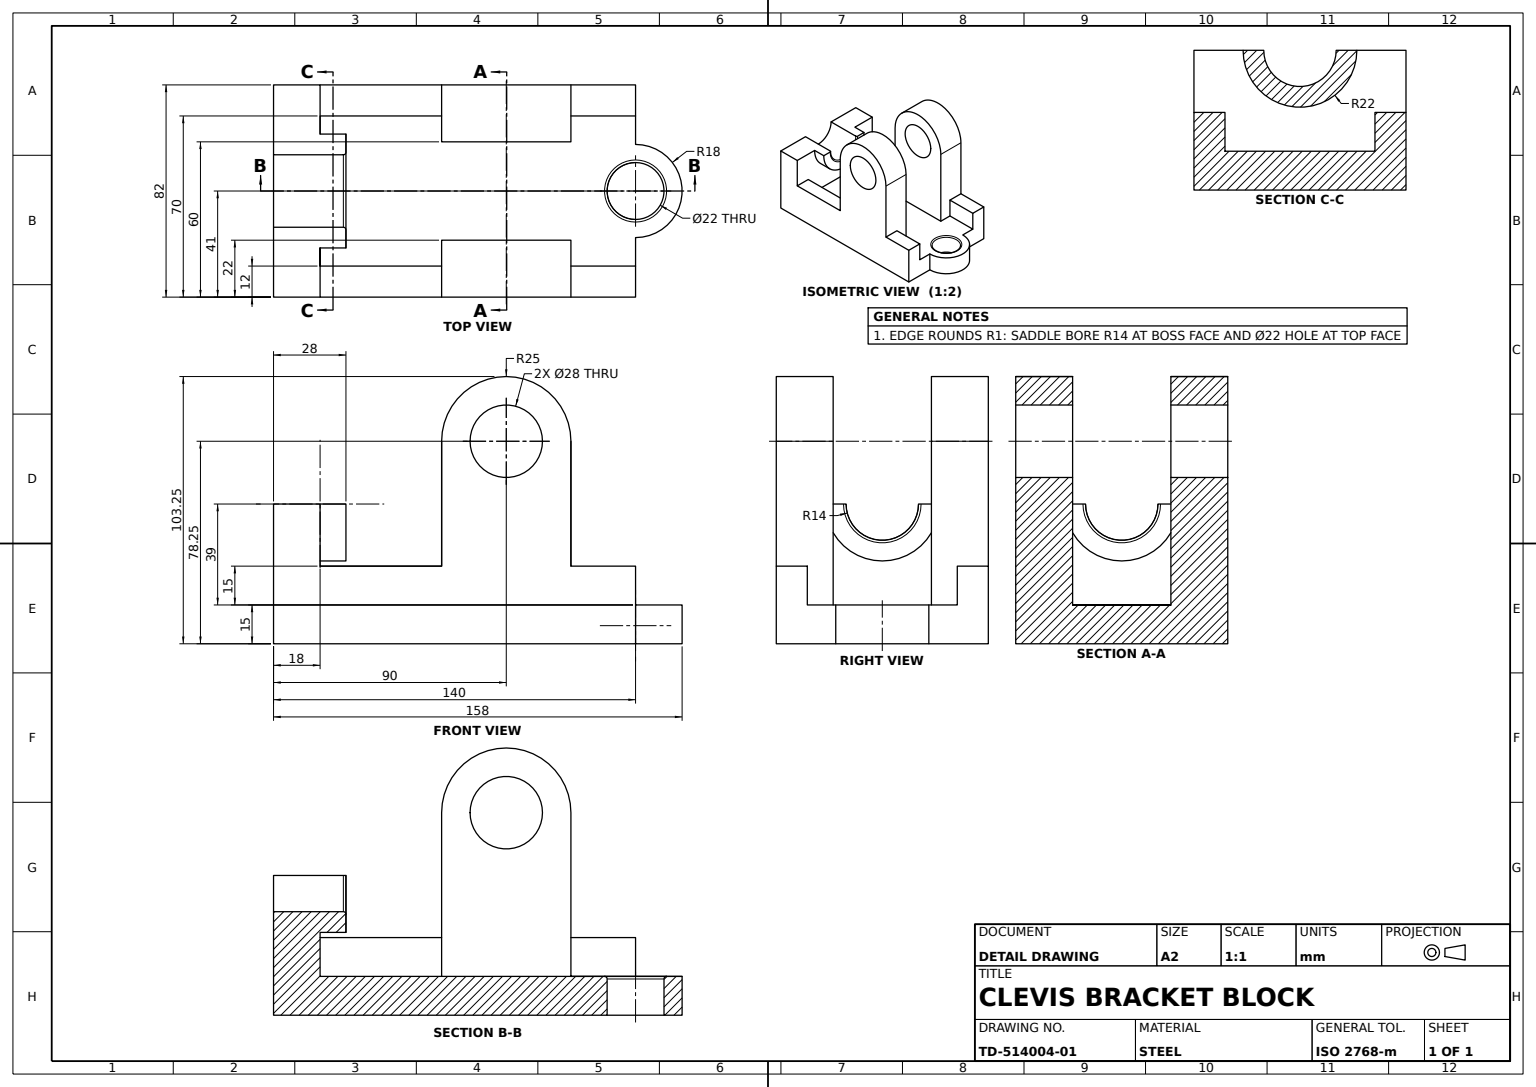
SolidWorks part; units mm, degrees
material "Plain Carbon Steel"
ref_plane "Front Plane" through (0, 0, 0) normal (0, 0, 1) x (1, 0, 0)
ref_plane "Top Plane" through (0, 0, 0) normal (0, 1, 0) x (1, 0, 0)
ref_plane "Right Plane" through (0, 0, 0) normal (1, 0, 0) x (0, 0, -1)
sketch "Base Plate Sketch" plane through (0, 0, 0) normal (0, 1, 0) x (1, 0, 0)
  line L0 (70, -18) -> (70, -41)
  line L1 (-70, 41) -> (70, 41)
  line L2 (-70, 41) -> (-70, -41)
  line L3 (-70, -41) -> (70, -41)
  line L4 (70, 41) -> (70, 18)
  line L5 (-70, 41) -> (70, -41) construction
  line L6 (-70, -41) -> (70, 41) construction
  arc A0 (70, -18) -> (70, 18) centre (70, 0) ccw
  circle A1 centre (70, 0) radius 11
  point P0 (0, 0)
  dimension "D3" = 36
  dimension "D4" = 22
  dimension "D1" = 82
  dimension "D2" = 140
  dimension "D5" = 23
  dimension "D6" = 41
extrude "Base Plate" add sketch "Base Plate Sketch" along normal blind 15
sketch "Rear Wall Sketch" plane through (0, 15, 0) normal (0, 1, 0) x (1, 0, 0)
  line L0 (-70, -41) -> (70, -41) construction
  line L1 (-70, 41) -> (-52, 41)
  line L2 (-70, 41) -> (-70, -41)
  line L3 (-70, -41) -> (-52, -41)
  line L4 (-52, 41) -> (-52, -41)
  dimension "D1" = 18
extrude "Rear Wall" add sketch "Rear Wall Sketch" along normal blind 39
sketch "Step Blocks Sketch" plane through (0, 15, 0) normal (0, 1, 0) x (1, 0, 0)
  line L0 (70, 18) -> (70, 41) construction
  line L1 (-52, 41) -> (70, 41)
  line L2 (-52, 41) -> (-52, 29)
  line L3 (-52, 29) -> (70, 29)
  line L4 (70, 41) -> (70, 29)
  line L5 (70, -41) -> (70, -18) construction
  line L6 (-52, -41) -> (70, -41)
  line L7 (-52, -41) -> (-52, -29)
  line L8 (-52, -29) -> (70, -29)
  line L9 (70, -41) -> (70, -29)
  dimension "D1" = 12
  dimension "D2" = 12
extrude "Step Blocks" add sketch "Step Blocks Sketch" along normal blind 15
sketch "Bearing Ear 1 Sketch" plane through (0, 0, 41) normal (0, 0, 1) x (1, 0, 0)
  line L0 (-70, 54) -> (-70, 0) construction
  line L4 (-5, 78.2548) -> (-5, 30)
  line L5 (-52, 30) -> (70, 30) construction
  line L6 (45, 78.2548) -> (45, 30)
  line L8 (-70, 0) -> (70, 0) construction
  line L9 (-5, 30) -> (-5, 0)
  line L10 (-5, 0) -> (45, 0)
  line L11 (45, 0) -> (45, 30)
  circle A0 centre (20, 78.2548) radius 14
  arc A1 (45, 78.2548) -> (-5, 78.2548) centre (20, 78.2548) ccw
  dimension "D1" = 28
  dimension "D2" = 50
  dimension "D3" = 90
  dimension "D4" = 78.2548
extrude "Bearing Ear 1" add sketch "Bearing Ear 1 Sketch" against normal blind 22
sketch "Bearing Ear 2 Sketch" plane through (0, 0, -41) normal (0, 0, -1) x (-1, 0, 0)
  line L0 (-45, 78.2548) -> (-45, 0)
  line L3 (-45, 0) -> (5, 0)
  line L4 (-70, 0) -> (70, 0) construction
  line L5 (5, 0) -> (5, 78.2548)
  circle A0 centre (-20, 78.2548) radius 14
  arc A1 (-45, 78.2548) -> (5, 78.2548) centre (-20, 78.2548) cw
  dimension "D1" = 25
  dimension "D2" = 28
  dimension "D3" = 78.2548
  dimension "D4" = 50
extrude "Bearing Ear 2" add sketch "Bearing Ear 2 Sketch" against normal blind 22
sketch "Saddle Cut Sketch" plane through (-70, 0, 0) normal (-1, 0, 0) x (0, 0, 1)
  line L0 (-41, 54) -> (41, 54) construction
  line L1 (-14, 54) -> (14, 54)
  arc A0 (-14, 54) -> (14, 54) centre (0, 54) ccw
  dimension "D1" = 14
extrude "Saddle Cut" cut sketch "Saddle Cut Sketch" against normal blind 22
sketch "Saddle Boss Sketch" plane through (-70, 0, 0) normal (-1, 0, 0) x (0, 0, 1)
  line L0 (-14, 54) -> (-22, 54)
  line L1 (14, 54) -> (22, 54)
  arc A0 (-22, 54) -> (22, 54) centre (0, 54) ccw
  arc A1 (-14, 54) -> (14, 54) centre (0, 54) ccw
  arc A2 (-14, 54) -> (14, 54) centre (0, 54) ccw construction
  dimension "D1" = 14
  dimension "D2" = 22
extrude "Saddle Boss" add sketch "Saddle Boss Sketch" against normal blind 28
fillet "Saddle Boss Fillet R1" radius 1 1 edges at (-42, 40, 0)
fillet "Base Edge Fillet R1" radius 1 1 edges at (70, 15, 11)
